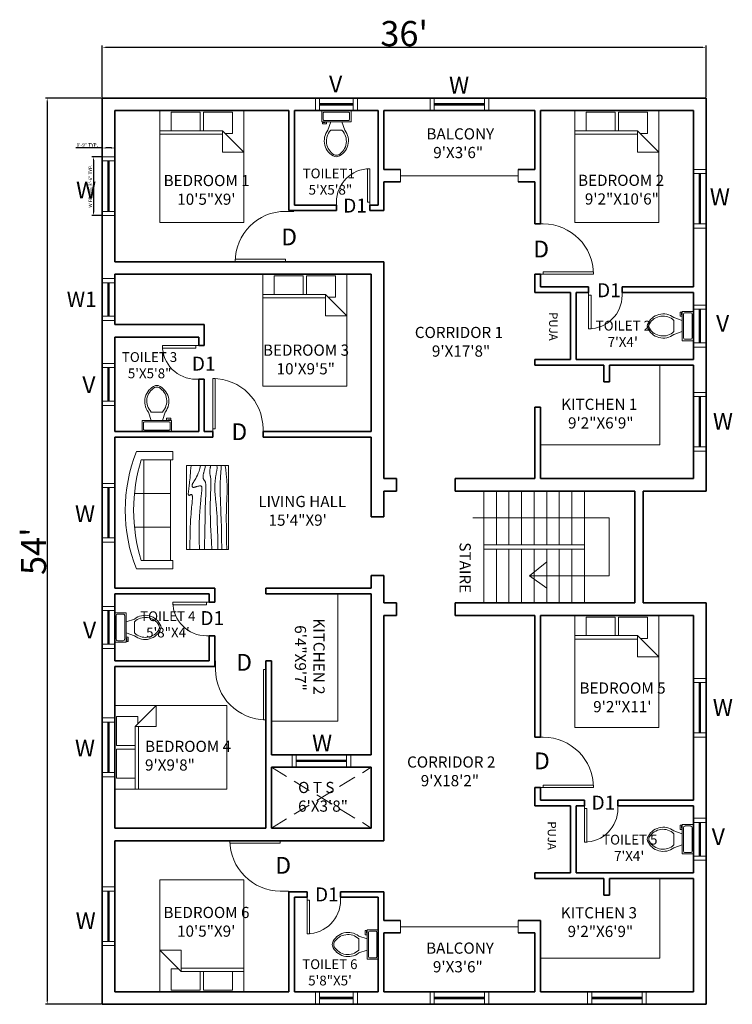
# Model space of a CAD drawing. Units: inches. Extents: x 2391 to 16591, y 7259 to 10239.
# Tile 18 of 27: x 3005 to 3515, y 8502 to 9206. Entities that reach past the tile are written whole.
import ezdxf

# ---------------------------------------------------------------- set-up
doc = ezdxf.new("R2010")
doc.units = ezdxf.units.IN
doc.linetypes.add('DASHED', pattern=[19.05, 12.7, -6.35])
for name, color, linetype, lineweight in [('A-ANNO-DIMS', 4, 'Continuous', 18), ('A-ANNO-IDEN', 2, 'Continuous', 18), ('A-ANNO-SYMB', 3, 'Continuous', 18), ('A-AREA-IDEN', 7, 'Continuous', 18), ('A-DOOR', 3, 'Continuous', 18), ('A-FLOR-CASE', 6, 'Continuous', 18), ('A-FLOR-FIXT', 9, 'Continuous', 18), ('A-FLOR-HRAL', 8, 'Continuous', 18), ('A-FLOR-OPEN', 4, 'DASHED', 13), ('A-FLOR-STRS', 7, 'Continuous', 18), ('A-FURN', 8, 'Continuous', 18), ('A-GLAZ', 4, 'Continuous', 18), ('A-WALL', 7, 'Continuous', 35)]:
    doc.layers.add(name, color=color, linetype=linetype, lineweight=lineweight)
doc.styles.get("Standard").update_dxf_attribs({"font": 'arial.ttf'})
doc.dimstyles.new('ISO-25', dxfattribs={"dimtxt": 2.5, "dimasz": 2.5, "dimexe": 1.25, "dimexo": 0.625, "dimtad": 1, "dimdec": 0, "dimlunit": 3, "dimtxsty": 'Standard', "dimcen": 2.5, "dimadec": 0, "dimazin": 0, "dimtfac": 1, "dimtdec": 0, "dimtmove": 0, "dimatfit": 3, "dimfxl": 1, "dimarcsym": 0})

# ---------------------------------------------------------------- blocks, each defined once
blk = doc.blocks.new('Bed - Queen')
for p, q in [((0, -80.00003), (0, 0)), ((0, 0), (59.99999, 0)), ((59.99999, 0), (59.99999, -80.00003)), ((7.99999, -1.2), (28.79998, -1.2)), ((7.99999, -14.4), (7.99999, -1.2)), ((28.79998, -1.2), (28.79998, -14.4)), ((31.19999, -1.2), (51.99999, -1.2)), ((31.19999, -14.4), (31.19999, -1.2)), ((51.99999, -1.2), (51.99999, -16.4)), ((0, -14.4), (44.8, -14.4)), ((44.8, -16.8), (0, -16.8)), ((59.99999, -29.6), (44.8, -14.4)), ((44.8, -14.4), (44.8, -29.6)), ((51.99999, -16.4), (46.79936, -16.4)), ((44.8, -29.6), (59.99999, -29.6)), ((59.99999, -80.00003), (0, -80.00003))]:
    blk.add_line(p, q)
blk = doc.blocks.new('Toilet - top')
for p, q in [((9.5, -6), (9.5, -2)), ((-10, -8.5), (-8, -8.5)), ((-10, -9.5), (-10, -8.5)), ((-7, -9.5), (-10, -9.5)), ((-8, -8.5), (-8, -8)), ((-7, -8), (-7, -9.5)), ((-4, -8), (-6, -14)), ((4, -14), (-4, -14)), ((4, -8), (6, -14))]:
    blk.add_line(p, q)
blk.add_lwpolyline([(10.5, -8), (10.5, 0), (-10.5, 0), (-10.5, -8)], close=True)
for points in [[(-9.5, -2), (-9.5, -6)], [(8.5, -1), (-8.5, -1)], [(-8.5, -7), (8.5, -7)]]:
    blk.add_lwpolyline(points)
for centre, radius, start, end in [((-8.62, -1.88), 0.884, 81.8699, 188.1301), ((-8.62, -6.12), 0.884, 171.8699, 278.1301), ((8.62, -1.88), 0.884, 351.8699, 98.1301), ((8.62, -6.12), 0.884, 261.8699, 8.1301), ((3.52, -21.58), 12.17, 141.46911, 247.97143), ((4.2, -21.82), 11.33, 136.36773, 238.94682), ((-3.52, -21.58), 12.17, 292.02843, 38.53071), ((-4.2, -21.82), 11.33, 301.05301, 43.63209), ((0, -27.88), 4, 245.73182, 294.26817), ((0, -29), 4, 254.86053, 285.13947)]:
    blk.add_arc(centre, radius, start, end)
blk = doc.blocks.new('Sofa - Roundback 7 ft.')
for p, q in [((-12.00002, -32.4421), (-12.00003, -6.5971)), ((11.99997, -32.4421), (11.99998, -6.5971)), ((-36.000027, -34), (-36.000027, -11.4696)), ((-35.999844, -13.3819), (35.9998, -13.3819)), ((35.99998, -34), (35.99998, -11.4696)), ((-36.000027, -32.4421), (35.99998, -32.4421))]:
    blk.add_line(p, q)
for points in [[(-36.000027, -34), (-42.000027, -34), (-42.000027, -8)], [(41.99998, -8), (41.99998, -34), (35.99998, -34)]]:
    blk.add_lwpolyline(points)
for centre, radius, start, end in [((0, -114.25), 114.25, 68.43141, 111.5686), ((-0.00001, -127.1968), 121.1968, 72.72033, 107.2797)]:
    blk.add_arc(centre, radius, start, end)
blk = doc.blocks.new('Table - Rectangular Woodgrain 60 x 30 in.')
for p, q in [((0, 0), (0, -30)), ((60, 0), (0, 0)), ((60, -30), (60, 0)), ((0, -30), (60, -30))]:
    blk.add_line(p, q)
for points in [[(0, -2.4), (4.8155, -2.418), (9.0302, -2.4688), (12.709, -2.5477), (15.9167, -2.65), (18.7181, -2.7711), (21.1781, -2.9063), (23.3616, -3.0508), (25.3333, -3.2), (27.1477, -3.3495), (28.8172, -3.4958), (30.3437, -3.636), (31.7291, -3.7667), (32.9756, -3.8849), (34.0849, -3.9875), (35.059, -4.0714), (35.9, -4.1334), (36.6114, -4.1711), (37.2041, -4.1854), (37.6906, -4.1779), (38.0833, -4.15), (38.3948, -4.1034), (38.6375, -4.0396), (38.8239, -3.9602), (38.9666, -3.8667), (39.0764, -3.7608), (39.1573, -3.6448), (39.2116, -3.521), (39.2416, -3.3917), (39.2498, -3.2593), (39.2385, -3.1261), (39.21, -2.9944), (39.1666, -2.8667), (39.111, -2.7447), (39.0468, -2.6281), (38.978, -2.5163), (38.9083, -2.4083), (38.8418, -2.3035), (38.7823, -2.201), (38.7337, -2.1001), (38.7, -2), (38.6844, -1.9003), (38.6875, -1.8021), (38.7094, -1.707), (38.75, -1.6167), (38.8094, -1.5326), (38.8875, -1.4563), (38.9844, -1.3893), (39.1, -1.3333), (39.2351, -1.2896), (39.3937, -1.2583), (39.5804, -1.2396), (39.8, -1.2333), (40.057, -1.2396), (40.3562, -1.2583), (40.7023, -1.2896), (41.1, -1.3333), (41.5547, -1.3895), (42.0755, -1.4573), (42.6721, -1.5361), (43.3542, -1.625), (44.1316, -1.7233), (45.014, -1.8302), (46.0114, -1.9449), (47.1333, -2.0667), (48.3862, -2.1947), (49.7625, -2.3281), (51.2513, -2.4663), (52.8416, -2.6083), (54.5226, -2.7535), (56.2833, -2.9011), (58.1127, -3.0501), (60, -3.2)], [(0, -9.2), (6.5759, -9.0858), (11.9385, -9.0365), (16.2527, -9.0418), (19.6833, -9.0917), (22.3952, -9.1759), (24.5531, -9.2844), (26.322, -9.4069), (27.8666, -9.5333), (29.3241, -9.6553), (30.7203, -9.7719), (32.0532, -9.8837), (33.3208, -9.9917), (34.5213, -10.0965), (35.6526, -10.199), (36.7128, -10.2999), (37.7, -10.4), (38.6129, -10.4996), (39.4531, -10.5969), (40.223, -10.6895), (40.925, -10.775), (41.5613, -10.8512), (42.1344, -10.9156), (42.6465, -10.966), (43.1, -11), (43.4976, -11.0158), (43.8437, -11.0136), (44.143, -10.9942), (44.4, -10.9583), (44.6195, -10.9069), (44.8062, -10.8406), (44.9648, -10.7603), (45.1, -10.6667), (45.2155, -10.5598), (45.3114, -10.4365), (45.3871, -10.2929), (45.4416, -10.125), (45.4743, -9.929), (45.4844, -9.7011), (45.4709, -9.4371), (45.4333, -9.1333), (45.3716, -8.7883), (45.2896, -8.4104), (45.1919, -8.0107), (45.0833, -7.6), (44.9685, -7.1893), (44.8521, -6.7896), (44.7388, -6.4117), (44.6333, -6.0667), (44.54, -5.7628), (44.4614, -5.4979), (44.4001, -5.2675), (44.3583, -5.0667), (44.3384, -4.8909), (44.3427, -4.7354), (44.3736, -4.5956), (44.4333, -4.4667), (44.5236, -4.3453), (44.6427, -4.2333), (44.7884, -4.1339), (44.9583, -4.05), (45.1501, -3.9849), (45.3614, -3.9417), (45.59, -3.9234), (45.8333, -3.9333), (46.0915, -3.9749), (46.3734, -4.0531), (46.6906, -4.1736), (47.0542, -4.3417), (47.4756, -4.5629), (47.9661, -4.8427), (48.5372, -5.1866), (49.2, -5.6), (49.9676, -6.0844), (50.8594, -6.625), (51.8965, -7.2031), (53.1, -7.8), (54.491, -8.3969), (56.0906, -8.975), (57.9199, -9.5156), (60, -10)], [(0, -12.8), (5.1847, -12.9322), (9.6213, -13.0323), (13.3963, -13.1059), (16.5958, -13.1583), (19.3063, -13.1952), (21.614, -13.2219), (23.6054, -13.2439), (25.3666, -13.2667), (26.9728, -13.2947), (28.4531, -13.3281), (29.8256, -13.3663), (31.1083, -13.4083), (32.3191, -13.4535), (33.476, -13.501), (34.597, -13.5501), (35.7, -13.6), (36.7984, -13.6497), (37.8875, -13.6979), (38.9578, -13.743), (40, -13.7833), (41.0047, -13.8174), (41.9625, -13.8438), (42.864, -13.8607), (43.7, -13.8667), (44.4631, -13.8604), (45.1552, -13.8417), (45.7801, -13.8104), (46.3416, -13.7667), (46.8439, -13.7104), (47.2906, -13.6417), (47.6858, -13.5604), (48.0333, -13.4667), (48.3375, -13.3608), (48.6042, -13.2448), (48.8396, -13.121), (49.05, -12.9917), (49.2417, -12.8593), (49.4208, -12.7261), (49.5937, -12.5944), (49.7667, -12.4667), (49.9452, -12.3451), (50.1323, -12.2313), (50.3303, -12.1268), (50.5416, -12.0333), (50.7686, -11.9524), (51.0135, -11.8854), (51.2788, -11.8341), (51.5666, -11.8), (51.8785, -11.7843), (52.2116, -11.7865), (52.562, -11.8059), (52.926, -11.8417), (53.2998, -11.8931), (53.6795, -11.9594), (54.0614, -12.0397), (54.4416, -12.1333), (54.8223, -12.2401), (55.2293, -12.3625), (55.6942, -12.5037), (56.2489, -12.6667), (56.9251, -12.8547), (57.7545, -13.0708), (58.7689, -13.3182), (60, -13.6)], [(0, -18), (5.124, -17.7273), (9.6609, -17.5057), (13.6705, -17.3303), (17.2125, -17.1958), (20.3467, -17.0973), (23.1328, -17.0297), (25.6307, -16.9878), (27.9, -16.9667), (29.9928, -16.9617), (31.9302, -16.9703), (33.7254, -16.9907), (35.3917, -17.0208), (36.9423, -17.0588), (38.3906, -17.1026), (39.7499, -17.1503), (41.0333, -17.2), (42.2519, -17.2496), (43.4073, -17.2969), (44.4986, -17.3395), (45.525, -17.375), (46.4858, -17.4012), (47.3802, -17.4156), (48.2074, -17.416), (48.9667, -17.4), (49.6583, -17.3662), (50.2872, -17.3167), (50.8595, -17.2547), (51.3812, -17.1833), (51.8584, -17.1057), (52.2971, -17.025), (52.7034, -16.9443), (53.0833, -16.8667), (53.443, -16.7951), (53.789, -16.7313), (54.128, -16.6768), (54.4666, -16.6334), (54.8115, -16.6024), (55.1693, -16.5854), (55.5465, -16.5841), (55.95, -16.6), (56.3828, -16.6337), (56.8346, -16.6823), (57.2915, -16.7418), (57.7396, -16.8084), (58.165, -16.878), (58.5539, -16.9469), (58.8924, -17.0111), (59.1666, -17.0667), (59.3679, -17.1107), (59.5078, -17.1438), (59.6032, -17.1675), (59.6708, -17.1833), (59.7275, -17.193), (59.7901, -17.1979), (59.8753, -17.1998), (60, -17.2)], [(0, -22.4), (8.0098, -22.2501), (14.4094, -22.1011), (19.4168, -21.9535), (23.25, -21.8083), (26.1269, -21.6663), (28.2656, -21.5281), (29.884, -21.3947), (31.2, -21.2667), (32.3967, -21.1448), (33.5172, -21.0292), (34.5697, -20.9198), (35.5625, -20.8167), (36.5037, -20.7198), (37.4015, -20.6292), (38.2642, -20.5448), (39.1, -20.4667), (39.9164, -20.3951), (40.7187, -20.3313), (41.5117, -20.2768), (42.3, -20.2333), (43.0883, -20.2024), (43.8812, -20.1854), (44.6836, -20.1841), (45.5, -20.2), (46.3328, -20.234), (47.1747, -20.2844), (48.0163, -20.3488), (48.8479, -20.425), (49.66, -20.5106), (50.4429, -20.6031), (51.1872, -20.7004), (51.8833, -20.8), (52.5246, -20.8999), (53.1166, -20.9995), (53.6681, -21.0983), (54.1875, -21.1958), (54.6834, -21.2919), (55.1646, -21.3859), (55.6394, -21.4777), (56.1167, -21.5667), (56.6028, -21.6515), (57.0961, -21.7266), (57.5929, -21.7852), (58.0896, -21.8208), (58.5823, -21.8268), (59.0674, -21.7964), (59.5412, -21.723), (60, -21.6)], [(0, -25.2), (8.6355, -25.0504), (15.7026, -24.9031), (21.4049, -24.7606), (25.9458, -24.625), (29.529, -24.4988), (32.3578, -24.3844), (34.6359, -24.284), (36.5667, -24.2), (38.3213, -24.1341), (39.9417, -24.0854), (41.437, -24.0523), (42.8167, -24.0333), (44.0901, -24.0268), (45.2667, -24.0313), (46.3557, -24.0451), (47.3667, -24.0667), (48.309, -24.0947), (49.1928, -24.1287), (50.0284, -24.168), (50.826, -24.2125), (51.5959, -24.2617), (52.3483, -24.3151), (53.0935, -24.3725), (53.8417, -24.4334), (54.6009, -24.497), (55.3699, -24.561), (56.1454, -24.6226), (56.9239, -24.6792), (57.7021, -24.7279), (58.4764, -24.7662), (59.2435, -24.7911), (60, -24.8)], [(0, -28.8), (5.6867, -28.6681), (10.45, -28.5698), (14.407, -28.5012), (17.675, -28.4584), (20.3711, -28.4374), (22.6125, -28.4344), (24.5164, -28.4455), (26.2, -28.4667), (27.762, -28.4947), (29.2276, -28.5281), (30.6033, -28.5663), (31.8958, -28.6084), (33.1118, -28.6535), (34.2578, -28.7011), (35.3405, -28.7501), (36.3666, -28.8), (37.3443, -28.8497), (38.288, -28.8974), (39.2137, -28.9412), (40.1375, -28.9792), (41.0753, -29.0093), (42.0432, -29.0297), (43.0572, -29.0384), (44.1333, -29.0333), (45.2936, -29.0114), (46.5843, -28.9641), (48.0579, -28.8816), (49.7666, -28.7542), (51.7629, -28.5721), (54.0989, -28.3255), (56.8272, -28.0048), (60, -27.6)]]:
    blk.add_lwpolyline(points)
blk = doc.blocks.new('*U7')
for p, q in [((0, 0), (0, -6)), ((36, 0), (36, -6))]:
    blk.add_line(p, q)
blk.add_lwpolyline([(0, 0), (0, 36), (1.75, 36), (1.75, 0)], close=True)
blk.add_arc((0, 0), 36, 0, 90)
blk = doc.blocks.new('*U6')
for p, q in [((-36, 0), (-36, 6)), ((0, 0), (0, 6))]:
    blk.add_line(p, q)
blk.add_lwpolyline([(0, 0), (0, -36), (-1.75, -36), (-1.75, 0)], close=True)
blk.add_arc((0, 0), 36, 180, 270)
blk = doc.blocks.new('*U8')
for p, q in [((-24, 0), (-24, -6)), ((0, 0), (0, -6))]:
    blk.add_line(p, q)
blk.add_lwpolyline([(0, 0), (0, 24), (-1.75, 24), (-1.75, 0)], close=True)
blk.add_arc((0, 0), 24, 90, 180)
blk = doc.blocks.new('*U9')
for p, q in [((0, 0), (0, 6)), ((24, 0), (24, 6))]:
    blk.add_line(p, q)
blk.add_lwpolyline([(0, 0), (0, -24), (1.75, -24), (1.75, 0)], close=True)
blk.add_arc((0, 0), 24, 270, 0)
blk = doc.blocks.new('*U10')
for p, q in [((0, 0), (0, -6)), ((-36, 0), (-36, -6))]:
    blk.add_line(p, q)
blk.add_lwpolyline([(0, 0), (0, 36), (-1.75, 36), (-1.75, 0)], close=True)
blk.add_arc((0, 0), 36, 90, 180)
blk = doc.blocks.new('*U11')
for p, q in [((-36, 0), (-36, 6)), ((0, 0), (0, 6))]:
    blk.add_line(p, q)
blk.add_lwpolyline([(0, 0), (0, -36), (-1.75, -36), (-1.75, 0)], close=True)
blk.add_arc((0, 0), 36, 180, 270)
blk = doc.blocks.new('*U12')
for p, q in [((0, 0), (0, -6)), ((-36, 0), (-36, -6))]:
    blk.add_line(p, q)
blk.add_lwpolyline([(0, 0), (0, 36), (-1.75, 36), (-1.75, 0)], close=True)
blk.add_arc((0, 0), 36, 90, 180)
blk = doc.blocks.new('*U13')
for p, q in [((0, 0), (0, 6)), ((36, 0), (36, 6))]:
    blk.add_line(p, q)
blk.add_lwpolyline([(0, 0), (0, -36), (1.75, -36), (1.75, 0)], close=True)
blk.add_arc((0, 0), 36, 270, 0)
blk = doc.blocks.new('*D23')
at = {"layer": 'A-ANNO-DIMS', "color": 0, "lineweight": -2, "transparency": 16777216}
for p, q in [((3064.34, 9150.16), (3064.34, 9187.06)), ((3066.84, 9185.81), (3493.84, 9185.81)), ((3496.34, 9150.16), (3496.34, 9187.06))]:
    blk.add_line(p, q, dxfattribs=at)
at = {"layer": 'A-ANNO-DIMS', "color": 0, "transparency": 16777216}
for points in [[(3066.84, 9186.23), (3066.84, 9185.4), (3064.34, 9185.81)], [(3493.84, 9186.23), (3493.84, 9185.4), (3496.34, 9185.81)]]:
    blk.add_solid(points, dxfattribs=at)
at = {"layer": 'Defpoints', "color": 0, "transparency": 16777216}
for p in [(3496.34, 9185.81), (3064.34, 9149.53), (3496.34, 9149.53)]:
    blk.add_point(p, dxfattribs=at)
at = {"layer": 'A-ANNO-DIMS', "color": 0, "transparency": 16777216, "insert": (3280.34, 9195.64), "char_height": 2.5, "attachment_point": 5}
blk.add_mtext("{\\H7.2x;36'}", dxfattribs=at)
blk = doc.blocks.new('*D24')
at = {"layer": 'A-ANNO-DIMS', "color": 0, "lineweight": -2, "transparency": 16777216}
for p, q in [((3063.71, 9149.53), (3023.67, 9149.53)), ((3024.92, 9147.03), (3024.92, 8504.03)), ((3063.71, 8501.53), (3023.67, 8501.53))]:
    blk.add_line(p, q, dxfattribs=at)
at = {"layer": 'A-ANNO-DIMS', "color": 0, "transparency": 16777216}
for points in [[(3024.5, 9147.03), (3025.34, 9147.03), (3024.92, 9149.53)], [(3024.5, 8504.03), (3025.34, 8504.03), (3024.92, 8501.53)]]:
    blk.add_solid(points, dxfattribs=at)
at = {"layer": 'Defpoints', "color": 0, "transparency": 16777216}
for p in [(3064.34, 9149.53), (3024.92, 8501.53), (3064.34, 8501.53)]:
    blk.add_point(p, dxfattribs=at)
at = {"layer": 'A-ANNO-DIMS', "color": 0, "transparency": 16777216, "insert": (3015.14, 8825.53), "char_height": 2.5, "attachment_point": 5, "rotation": 90}
blk.add_mtext("{\\H7.2x;54'}", dxfattribs=at)
blk = doc.blocks.new('WINDOW-36-PLAN')
for p, q in [((9, 42), (0, 42)), ((9, 39), (0, 39)), ((4, 39), (4, 3)), ((4.5, 39), (4.5, 3)), ((5, 39), (5, 3)), ((9, 3), (0, 3)), ((9, 0), (0, 0))]:
    blk.add_line(p, q)
blk = doc.blocks.new('VENT-24-PLAN')
for p, q in [((9, 30), (0, 30)), ((9, 27), (0, 27)), ((4, 27), (4, 3)), ((4.5, 27), (4.5, 3)), ((5, 27), (5, 3)), ((9, 3), (0, 3)), ((9, 0), (0, 0))]:
    blk.add_line(p, q)
blk = doc.blocks.new('WINDOW-24-PLAN')
for p, q in [((9, 30), (0, 30)), ((9, 27), (0, 27)), ((4, 27), (4, 3)), ((4.5, 27), (4.5, 3)), ((5, 27), (5, 3)), ((9, 3), (0, 3)), ((9, 0), (0, 0))]:
    blk.add_line(p, q)
blk = doc.blocks.new('STAIR-RETURN-FLIGHT')
for p, q in [((0, 80), (0, 0)), ((9, 80), (9, 41.5)), ((18, 80), (18, 41.5)), ((27, 80), (27, 41.5)), ((36, 80), (36, 41.5)), ((45, 80), (45, 41.5)), ((54, 80), (54, 41.5)), ((63, 80), (63, 41.5)), ((72, 80), (72, 0)), ((72, 41.5), (0, 41.5)), ((72, 38.5), (0, 38.5)), ((9, 38.5), (9, 0)), ((18, 38.5), (18, 0)), ((27, 38.5), (27, 0)), ((36, 38.5), (36, 0)), ((45, 38.5), (45, 0)), ((54, 38.5), (54, 0)), ((63, 38.5), (63, 0))]:
    blk.add_line(p, q)
blk = doc.blocks.new('STAIR-DIRECTION-ARROW')
for p, q in [((0, 50.31), (97.37, 50.31)), ((97.37, 50.31), (97.37, 8.81)), ((40.34, 8.81), (52.74, 18.89)), ((97.37, 8.81), (40.34, 8.81)), ((40.34, 8.81), (52.74, 0))]:
    blk.add_line(p, q)
blk = doc.blocks.new('COUNTER-L-RETURN')
for q in [(47.5, 91), (0, 0)]:
    blk.add_line((47.5, 0), q)
blk = doc.blocks.new('COUNTER-L-KITCHEN')
for p, q in [((85.5, 57), (85.5, 0)), ((85.5, 0), (0, 0))]:
    blk.add_line(p, q)
blk = doc.blocks.new('*D39')
at = {"layer": 'A-ANNO-DIMS', "color": 0, "lineweight": -2, "transparency": 16777216}
for p, q in [((3063.71, 9107.53), (3056.79, 9107.53)), ((3058.04, 9105.03), (3058.04, 9068.03)), ((3063.71, 9065.53), (3056.79, 9065.53))]:
    blk.add_line(p, q, dxfattribs=at)
at = {"layer": 'A-ANNO-DIMS', "color": 0, "transparency": 16777216}
for points in [[(3057.62, 9105.03), (3058.46, 9105.03), (3058.04, 9107.53)], [(3057.62, 9068.03), (3058.46, 9068.03), (3058.04, 9065.53)]]:
    blk.add_solid(points, dxfattribs=at)
at = {"layer": 'Defpoints', "color": 0, "transparency": 16777216}
for p in [(3064.34, 9107.53), (3058.04, 9065.53), (3064.34, 9065.53)]:
    blk.add_point(p, dxfattribs=at)
at = {"layer": 'A-ANNO-DIMS', "color": 0, "transparency": 16777216, "insert": (3056.14, 9086.53), "char_height": 2.5, "attachment_point": 5, "rotation": 90}
blk.add_mtext('W FRAME 3\'-6" TYP.', dxfattribs=at)
blk = doc.blocks.new('*D40')
at = {"layer": 'A-ANNO-DIMS', "color": 0, "lineweight": -2, "transparency": 16777216}
for p, q in [((3064.34, 9113.83), (3045.35, 9113.83)), ((3064.34, 9108.16), (3064.34, 9115.08)), ((3070.84, 9113.83), (3066.84, 9113.83)), ((3073.34, 9108.16), (3073.34, 9115.08))]:
    blk.add_line(p, q, dxfattribs=at)
at = {"layer": 'A-ANNO-DIMS', "color": 0, "transparency": 16777216}
for points in [[(3066.84, 9114.25), (3066.84, 9113.41), (3064.34, 9113.83)], [(3070.84, 9114.25), (3070.84, 9113.41), (3073.34, 9113.83)]]:
    blk.add_solid(points, dxfattribs=at)
at = {"layer": 'Defpoints', "color": 0, "transparency": 16777216}
for p in [(3064.34, 9113.83), (3064.34, 9107.53), (3073.34, 9107.53)]:
    blk.add_point(p, dxfattribs=at)
at = {"layer": 'A-ANNO-DIMS', "color": 0, "transparency": 16777216, "insert": (3053.6, 9115.73), "char_height": 2.5, "attachment_point": 5}
blk.add_mtext('0\'-9" TYP.', dxfattribs=at)

msp = doc.modelspace()

# ---------------------------------------------------------------- linework, layer by layer
at = {"layer": 'A-DOOR'}
msp.add_line((3197.69, 8618.53), (3197.69, 8618.53), dxfattribs=at)
at = {"layer": 'A-FLOR-HRAL'}
for p, q in [((3277.84, 9089.53), (3277.84, 9098.53)), ((3361.84, 9089.53), (3361.84, 9098.53)), ((3277.84, 9094.03), (3361.84, 9094.03)), ((3277.84, 8552.53), (3277.84, 8561.53)), ((3361.84, 8552.53), (3361.84, 8561.53)), ((3277.84, 8557.03), (3361.84, 8557.03))]:
    msp.add_line(p, q, dxfattribs=at)
at = {"layer": 'A-FLOR-OPEN'}
for p, q in [((3185.34, 8627.53), (3256.84, 8671.03)), ((3185.34, 8671.03), (3256.84, 8627.53))]:
    msp.add_line(p, q, dxfattribs=at)
at = {"layer": 'A-WALL'}
for p, q in [((3064.34, 9149.53), (3496.34, 9149.53)), ((3064.34, 8501.53), (3064.34, 9149.53)), ((3496.34, 9149.53), (3496.34, 8868.53)), ((3073.34, 9140.53), (3197.84, 9140.53)), ((3073.34, 9032.53), (3073.34, 9140.53)), ((3197.84, 9069.03), (3197.84, 9140.53)), ((3201.84, 9140.53), (3261.84, 9140.53)), ((3201.84, 9073.03), (3201.84, 9140.53)), ((3261.84, 9073.03), (3261.84, 9140.53)), ((3265.84, 9140.53), (3373.84, 9140.53)), ((3265.84, 9098.53), (3265.84, 9140.53)), ((3373.84, 9098.53), (3373.84, 9140.53)), ((3377.84, 9140.53), (3487.34, 9140.53)), ((3377.84, 9059.53), (3377.84, 9140.53)), ((3487.34, 9140.53), (3487.34, 9014.53)), ((3265.84, 9098.53), (3277.84, 9098.53)), ((3361.84, 9098.53), (3373.84, 9098.53)), ((3265.84, 9089.53), (3277.84, 9089.53)), ((3265.84, 9069.03), (3265.84, 9089.53)), ((3361.84, 9089.53), (3373.84, 9089.53)), ((3373.84, 9059.53), (3373.84, 9089.53)), ((3197.84, 9069.03), (3231.84, 9069.03)), ((3201.84, 9073.03), (3231.84, 9073.03)), ((3231.84, 9069.03), (3231.84, 9073.03)), ((3255.84, 9073.03), (3261.84, 9073.03)), ((3255.84, 9069.03), (3255.84, 9073.03)), ((3255.84, 9069.03), (3265.84, 9069.03)), ((3373.84, 9059.53), (3377.84, 9059.53)), ((3073.34, 9032.53), (3265.84, 9032.53)), ((3265.84, 8877.53), (3265.84, 9032.53)), ((3073.34, 9023.53), (3256.84, 9023.53)), ((3073.34, 8987.53), (3073.34, 9023.53)), ((3256.84, 8911.03), (3256.84, 9023.53)), ((3373.84, 9023.53), (3377.84, 9023.53)), ((3373.84, 9010.53), (3373.84, 9023.53)), ((3377.84, 9014.53), (3377.84, 9023.53)), ((3377.84, 9014.53), (3412.34, 9014.53)), ((3412.34, 9014.53), (3412.34, 9010.53)), ((3436.34, 9014.53), (3487.34, 9014.53)), ((3436.34, 9014.53), (3436.34, 9010.53)), ((3373.84, 9010.53), (3399.34, 9010.53)), ((3399.34, 9010.53), (3399.34, 8962.53)), ((3403.34, 9010.53), (3412.34, 9010.53)), ((3403.34, 9010.53), (3403.34, 8962.53)), ((3436.34, 9010.53), (3487.34, 9010.53)), ((3487.34, 9010.53), (3487.34, 8962.53)), ((3073.34, 8987.53), (3137.34, 8987.53)), ((3137.34, 8972.53), (3137.34, 8987.53)), ((3073.34, 8978.53), (3133.34, 8978.53)), ((3073.34, 8911.03), (3073.34, 8978.53)), ((3133.34, 8972.53), (3133.34, 8978.53)), ((3133.34, 8972.53), (3137.34, 8972.53)), ((3373.84, 8962.53), (3399.34, 8962.53)), ((3373.84, 8958.53), (3373.84, 8962.53)), ((3403.34, 8962.53), (3487.34, 8962.53)), ((3373.84, 8958.53), (3423.34, 8958.53)), ((3423.34, 8958.53), (3423.34, 8946.53)), ((3427.34, 8958.53), (3487.34, 8958.53)), ((3427.34, 8958.53), (3427.34, 8946.53)), ((3487.34, 8958.53), (3487.34, 8877.53)), ((3133.34, 8948.53), (3137.34, 8948.53)), ((3133.34, 8911.03), (3133.34, 8948.53)), ((3137.34, 8911.03), (3137.34, 8948.53)), ((3423.34, 8946.53), (3427.34, 8946.53)), ((3373.84, 8928.53), (3377.84, 8928.53)), ((3373.84, 8877.53), (3373.84, 8928.53)), ((3377.84, 8877.53), (3377.84, 8928.53)), ((3073.34, 8911.03), (3133.34, 8911.03)), ((3073.34, 8907.03), (3143.34, 8907.03)), ((3073.34, 8799.03), (3073.34, 8907.03)), ((3137.34, 8911.03), (3143.34, 8911.03)), ((3143.34, 8907.03), (3143.34, 8911.03)), ((3179.34, 8911.03), (3256.84, 8911.03)), ((3179.34, 8907.03), (3179.34, 8911.03)), ((3179.34, 8907.03), (3256.84, 8907.03)), ((3256.84, 8850.03), (3256.84, 8907.03)), ((3265.84, 8877.53), (3274.84, 8877.53)), ((3274.84, 8868.53), (3274.84, 8877.53)), ((3316.84, 8877.53), (3373.84, 8877.53)), ((3316.84, 8868.53), (3316.84, 8877.53)), ((3377.84, 8877.53), (3487.34, 8877.53)), ((3265.84, 8868.53), (3274.84, 8868.53)), ((3265.84, 8850.03), (3265.84, 8868.53)), ((3316.84, 8868.53), (3445.34, 8868.53)), ((3445.34, 8868.53), (3445.34, 8788.53)), ((3451.34, 8868.53), (3496.34, 8868.53)), ((3451.34, 8868.53), (3451.34, 8788.53)), ((3256.84, 8850.03), (3265.84, 8850.03)), ((3256.84, 8808.03), (3265.84, 8808.03)), ((3256.84, 8799.03), (3256.84, 8808.03)), ((3265.84, 8788.53), (3265.84, 8808.03)), ((3073.34, 8799.03), (3144.84, 8799.03)), ((3073.34, 8795.03), (3140.84, 8795.03)), ((3073.34, 8747.03), (3073.34, 8795.03)), ((3140.84, 8789.03), (3140.84, 8795.03)), ((3144.84, 8789.03), (3144.84, 8799.03)), ((3181.34, 8799.03), (3256.84, 8799.03)), ((3181.34, 8795.03), (3181.34, 8799.03)), ((3181.34, 8795.03), (3256.84, 8795.03)), ((3256.84, 8680.03), (3256.84, 8795.03)), ((3140.84, 8789.03), (3144.84, 8789.03)), ((3274.84, 8788.53), (3265.84, 8788.53)), ((3274.84, 8779.53), (3274.84, 8788.53)), ((3445.34, 8788.53), (3316.84, 8788.53)), ((3316.84, 8779.53), (3316.84, 8788.53)), ((3496.34, 8788.53), (3451.34, 8788.53)), ((3496.34, 8788.53), (3496.34, 8501.53)), ((3274.84, 8779.53), (3265.84, 8779.53)), ((3265.84, 8618.53), (3265.84, 8779.53)), ((3373.84, 8779.53), (3316.84, 8779.53)), ((3373.84, 8692.53), (3373.84, 8779.53)), ((3487.34, 8779.53), (3377.84, 8779.53)), ((3377.84, 8692.53), (3377.84, 8779.53)), ((3487.34, 8779.53), (3487.34, 8647.53)), ((3140.84, 8765.03), (3144.84, 8765.03)), ((3140.84, 8747.03), (3140.84, 8765.03)), ((3144.84, 8743.03), (3144.84, 8765.03)), ((3073.34, 8747.03), (3140.84, 8747.03)), ((3181.34, 8747.03), (3185.34, 8747.03)), ((3181.34, 8627.53), (3181.34, 8747.03)), ((3185.34, 8680.03), (3185.34, 8747.03)), ((3073.34, 8743.03), (3144.84, 8743.03)), ((3073.34, 8627.53), (3073.34, 8743.03)), ((3377.84, 8692.53), (3373.84, 8692.53)), ((3256.84, 8680.03), (3185.34, 8680.03)), ((3256.84, 8671.03), (3185.34, 8671.03)), ((3185.34, 8627.53), (3185.34, 8671.03)), ((3256.84, 8627.53), (3256.84, 8671.03)), ((3377.84, 8656.53), (3373.84, 8656.53)), ((3373.84, 8643.53), (3373.84, 8656.53)), ((3377.84, 8647.53), (3377.84, 8656.53)), ((3409.34, 8647.53), (3377.84, 8647.53)), ((3409.34, 8647.53), (3409.34, 8643.53)), ((3433.34, 8647.53), (3433.34, 8643.53)), ((3487.34, 8647.53), (3433.34, 8647.53)), ((3399.34, 8643.53), (3373.84, 8643.53)), ((3399.34, 8643.53), (3399.34, 8595.53)), ((3403.34, 8643.53), (3403.34, 8595.53)), ((3409.34, 8643.53), (3403.34, 8643.53)), ((3487.34, 8643.53), (3433.34, 8643.53)), ((3487.34, 8643.53), (3487.34, 8595.53)), ((3181.34, 8627.53), (3073.34, 8627.53)), ((3256.84, 8627.53), (3185.34, 8627.53)), ((3201.84, 8618.53), (3073.34, 8618.53)), ((3073.34, 8510.53), (3073.34, 8618.53)), ((3265.84, 8618.53), (3201.84, 8618.53)), ((3399.34, 8595.53), (3373.84, 8595.53)), ((3373.84, 8591.53), (3373.84, 8595.53)), ((3423.34, 8591.53), (3373.84, 8591.53)), ((3487.34, 8595.53), (3403.34, 8595.53)), ((3423.34, 8591.53), (3423.34, 8579.53)), ((3427.34, 8591.53), (3427.34, 8579.53)), ((3487.34, 8591.53), (3427.34, 8591.53)), ((3487.34, 8591.53), (3487.34, 8510.53)), ((3210.84, 8582.03), (3197.84, 8582.03)), ((3197.84, 8510.53), (3197.84, 8582.03)), ((3210.84, 8578.03), (3201.84, 8578.03)), ((3201.84, 8510.53), (3201.84, 8578.03)), ((3210.84, 8578.03), (3210.84, 8582.03)), ((3265.84, 8582.03), (3234.84, 8582.03)), ((3234.84, 8578.03), (3234.84, 8582.03)), ((3261.84, 8578.03), (3234.84, 8578.03)), ((3261.84, 8510.53), (3261.84, 8578.03)), ((3265.84, 8561.53), (3265.84, 8582.03)), ((3427.34, 8579.53), (3423.34, 8579.53)), ((3277.84, 8561.53), (3265.84, 8561.53)), ((3377.84, 8561.53), (3361.84, 8561.53)), ((3377.84, 8510.53), (3377.84, 8561.53)), ((3277.84, 8552.53), (3265.84, 8552.53)), ((3265.84, 8510.53), (3265.84, 8552.53)), ((3373.84, 8552.53), (3361.84, 8552.53)), ((3373.84, 8510.53), (3373.84, 8552.53)), ((3197.84, 8510.53), (3073.34, 8510.53)), ((3261.84, 8510.53), (3201.84, 8510.53)), ((3373.84, 8510.53), (3265.84, 8510.53)), ((3487.34, 8510.53), (3377.84, 8510.53)), ((3496.34, 8501.53), (3064.34, 8501.53))]:
    msp.add_line(p, q, dxfattribs=at)

# ---------------------------------------------------------------- block references
at = {"layer": 'A-ANNO-SYMB'}
msp.add_blockref('STAIR-DIRECTION-ARROW', (3329.6, 8798.98), dxfattribs=at)
at = {"layer": 'A-DOOR'}
for name, p in [('*U8', (3255.84, 9075.03)), ('*U9', (3412.34, 9008.53)), ('*U7', (3143.34, 8913.03)), ('*U6', (3181.34, 8741.03)), ('*U9', (3409.34, 8641.53)), ('*U9', (3210.84, 8576.03))]:
    msp.add_blockref(name, p, dxfattribs=at)
at = {"layer": 'A-DOOR', "rotation": 270}
for name, p in [('*U11', (3195.44, 9032.53)), ('*U12', (3379.84, 9023.53)), ('*U9', (3131.34, 8972.53)), ('*U9', (3138.84, 8789.03)), ('*U10', (3379.84, 8656.53)), ('*U13', (3191.69, 8618.53))]:
    msp.add_blockref(name, p, dxfattribs=at)
at = {"layer": 'A-FLOR-CASE'}
for name, p in [('COUNTER-L-KITCHEN', (3377.84, 8901.53)), ('COUNTER-L-RETURN', (3185.34, 8704.03)), ('COUNTER-L-KITCHEN', (3377.84, 8534.53))]:
    msp.add_blockref(name, p, dxfattribs=at)
at = {"layer": 'A-FLOR-FIXT'}
msp.add_blockref('Toilet - top', (3231.84, 9140.53), dxfattribs=at)
for p, rotation in [((3487.34, 8986.53), 270), ((3103.34, 8911.03), 180), ((3073.34, 8771.03), 89.99999999999999), ((3487.34, 8619.53), 270), ((3261.84, 8544.28), 270)]:
    msp.add_blockref('Toilet - top', p, dxfattribs=dict(at, rotation=rotation))
at = {"layer": 'A-FLOR-STRS', "rotation": 180}
msp.add_blockref('STAIR-RETURN-FLIGHT', (3409.34, 8868.53), dxfattribs=at)
at = {"layer": 'A-FURN'}
for p in [(3105.59, 9140.53), (3402.59, 9140.53), (3179.31, 9023.53), (3402.59, 8779.53)]:
    msp.add_blockref('Bed - Queen', p, dxfattribs=at)
for name, p, rotation in [('Sofa - Roundback 7 ft.', (3080.73, 8854.81), 90), ('Table - Rectangular Woodgrain 60 x 30 in.', (3124.64, 8826.76), 90), ('Bed - Queen', (3073.34, 8655.28), 90), ('Bed - Queen', (3165.59, 8510.53), 180)]:
    msp.add_blockref(name, p, dxfattribs=dict(at, rotation=rotation))
at = {"layer": 'A-GLAZ'}
for name, p, rotation in [('VENT-24-PLAN', (3246.84, 9140.53), 90.0000000000009), ('WINDOW-36-PLAN', (3340.84, 9140.53), 90.00000000000396), ('WINDOW-36-PLAN', (3073.34, 9107.53), 180), ('WINDOW-36-PLAN', (3496.34, 9098.53), 180), ('WINDOW-24-PLAN', (3073.34, 9020.53), 180), ('VENT-24-PLAN', (3496.34, 9001.53), 180), ('VENT-24-PLAN', (3073.34, 8959.78), 180), ('WINDOW-36-PLAN', (3496.34, 8939.03), 180), ('WINDOW-36-PLAN', (3073.34, 8874.03), 180), ('VENT-24-PLAN', (3073.34, 8786.03), 180), ('WINDOW-36-PLAN', (3496.34, 8734.53), 180), ('WINDOW-36-PLAN', (3073.34, 8706.28), 180), ('WINDOW-36-PLAN', (3242.09, 8671.03), 90.00000000000423), ('VENT-24-PLAN', (3496.34, 8634.53), 180), ('WINDOW-36-PLAN', (3073.34, 8585.53), 180), ('VENT-24-PLAN', (3246.84, 8501.53), 90.0000000000009), ('WINDOW-36-PLAN', (3340.84, 8501.53), 90.00000000000003), ('WINDOW-36-PLAN', (3453.59, 8501.53), 89.99999999999976)]:
    msp.add_blockref(name, p, dxfattribs=dict(at, rotation=rotation))

# ---------------------------------------------------------------- texts
at = {"layer": 'A-ANNO-IDEN', "attachment_point": 1}
for s, width, insert, char_height in [('V', 33.2285, (3226.61, 9165.53), 12), ('W', 41.0391, (3312.46, 9164.73), 12), ('W', 25.6098, (3045.56, 9089.72), 12), ('W', 63.2637, (3499.07, 9084.88), 12), ('D1', 88.0557, (3236.74, 9077.64), 10), ('D', 711.4851, (3192.39, 9056.24), 12), ('D', 1570.4564, (3372.75, 9047.55), 12), ('D1', 69.9915, (3418.39, 9017.11), 10), ('W1', 26.8712, (3038.89, 9011.17), 11), ('V', 60.3219, (3503.54, 8994.49), 12), ('D1', 74.2476, (3128.42, 8964.63), 10), ('V', 17.0712, (3050.03, 8950.59), 12), ('W', 105.2929, (3501.24, 8924.44), 12), ('D ', 382.5297, (3156.75, 8916.92), 12), ('W', 40.7205, (3044.77, 8858.35), 12), ('D1', 102.8831, (3134.54, 8782.67), 10), ('V', 16.5796, (3050.52, 8775.11), 12), ('D', 433.7706, (3160.16, 8752.05), 12), ('W', 123.7268, (3501.2, 8719.74), 12), ('W', 28.3648, (3044.75, 8690.78), 12), ('W', 47.6363, (3214.43, 8694.41), 12), ('D', 235.1744, (3373.29, 8681.59), 12), ('D1', 70.0055, (3414.45, 8650.73), 10), ('V', 48.5524, (3500.45, 8627.33), 12), ('D', 460.223, (3188.15, 8606.89), 12), ('D1', 90.0045, (3216.54, 8585.09), 10), ('W', 32.8374, (3045.27, 8567.27), 12)]:
    msp.add_mtext_dynamic_manual_height_columns(s, width=width, gutter_width=12.5, heights=[0], dxfattribs=dict(at, insert=insert, char_height=char_height))
at = {"layer": 'A-AREA-IDEN', "attachment_point": 1}
for s, width, insert, char_height in [('BALCONY\\P  9\'X3\'6"', 125.309, (3296.28, 9127.91), 8), ('TOILET1\\P  5\'X5\'8"', 175.2431, (3207.68, 9099.14), 7), ('BEDROOM 1\\P    10\'5"X9\'', 152.4027, (3108.19, 9094.55), 8), ('BEDROOM 2\\P  9\'2"X10\'6"', 186.7643, (3404.76, 9094.72), 8), ('CORRIDOR 1\\P     9\'X17\'8"', 386.0733, (3287.97, 8985.94), 8), ("{\\H0.875x;TOILET 2\\P    7'X4}'", 130.8261, (3417.42, 8990.3), 8), ('BEDROOM 3\\P    10\'X9\'5"', 134.4574, (3179.31, 8973.29), 8), ('TOILET 3\\P  5\'X5\'8"', 110.3725, (3078.34, 8967.85), 7), ('KITCHEN 1\\P  9\'2"X6\'9"', 260.4884, (3392.71, 8934.57), 8), ('LIVING HALL\\P   15\'4"X9\'', 316.1653, (3175.97, 8865.07), 8), ('TOILET 4\\P  5\'8"X4\'', 115.6049, (3091.42, 8782.53), 7), ('BEDROOM 5\\P    9\'2"X11\'', 234.3403, (3405.83, 8731.68), 8), ('BEDROOM 4\\P9\'X9\'8"', 337.9313, (3094.9, 8689.98), 8), ('CORRIDOR 2\\P    9\'X18\'2"  ', 260.1533, (3282.44, 8678.78), 8), ('O T S\\P6\'X3\'8"', 143.5906, (3204.45, 8660.58), 8), ("{\\H0.875x;TOILET 5\\P    7'X4}'", 130.8261, (3422.02, 8622.76), 8), ('BEDROOM 6\\P    10\'5"X9\'', 279.7405, (3108.07, 8571.2), 8), ('KITCHEN 3\\P  9\'2"X6\'9"', 205.0668, (3392.43, 8570.98), 8), ('BALCONY\\P  9\'X3\'6"', 151.3379, (3296.03, 8545.72), 8), ('TOILET 6\\P  5\'8"X5\'', 210.0226, (3207.4, 8533.7), 7)]:
    msp.add_mtext_dynamic_manual_height_columns(s, width=width, gutter_width=12.5, heights=[0], dxfattribs=dict(at, insert=insert, char_height=char_height))
at = {"layer": 'A-AREA-IDEN', "attachment_point": 1, "rotation": 270}
for s, width, insert, char_height in [('PUJA', 212.5876, (3390.1, 8996.5), 6), ('STAIRE', 212.5876, (3328.01, 8831.83), 8), ('KITCHEN 2\\P  6\'4"X9\'7"', 154.6668, (3223.45, 8777.49), 8), ('PUJA', 212.5876, (3389.08, 8632.37), 6)]:
    msp.add_mtext_dynamic_manual_height_columns(s, width=width, gutter_width=12.5, heights=[0], dxfattribs=dict(at, insert=insert, char_height=char_height))

# ---------------------------------------------------------------- dimensions: what is measured, and where the dimension line sits
at = {"layer": 'A-ANNO-DIMS'}
dim = msp.add_linear_dim(base=(3496.34, 9185.81), p1=(3064.34, 9149.53), p2=(3496.34, 9149.53), text='{\\H7.2x;<>}', dimstyle='ISO-25', override={"dimclrd": 0, "dimclre": 0, "dimclrt": 0}, dxfattribs=at)
dim.commit()
dim.dimension.update_dxf_attribs({"geometry": '*D23', "text_midpoint": (3280.34, 9195.64)})
for base, p1, p2, angle, text, override, picture, middle in [((3024.92, 8501.53), (3064.34, 9149.53), (3064.34, 8501.53), 90, '{\\H7.2x;<>}', {"dimclrd": 0, "dimclre": 0, "dimclrt": 0}, '*D24', (3015.14, 8825.53)), ((3064.34, 9113.83), (3073.34, 9107.53), (3064.34, 9107.53), 180, '<> TYP.', {"dimdec": 1, "dimlfac": 1, "dimrnd": 0, "dimzin": 1, "dimdsep": 46, "dimlunit": 4, "dimfrac": 2}, '*D40', (3053.6, 9115.73)), ((3058.04, 9065.53), (3064.34, 9107.53), (3064.34, 9065.53), 270, 'W FRAME <> TYP.', {"dimdec": 1, "dimlfac": 1, "dimrnd": 0, "dimzin": 1, "dimdsep": 46, "dimlunit": 4, "dimfrac": 2}, '*D39', (3056.14, 9086.53))]:
    dim = msp.add_linear_dim(base=base, p1=p1, p2=p2, angle=angle, text=text, dimstyle='ISO-25', override=override, dxfattribs=at)
    dim.commit()
    dim.dimension.update_dxf_attribs({"geometry": picture, "text_midpoint": middle})

doc.saveas('drawing.dxf')
